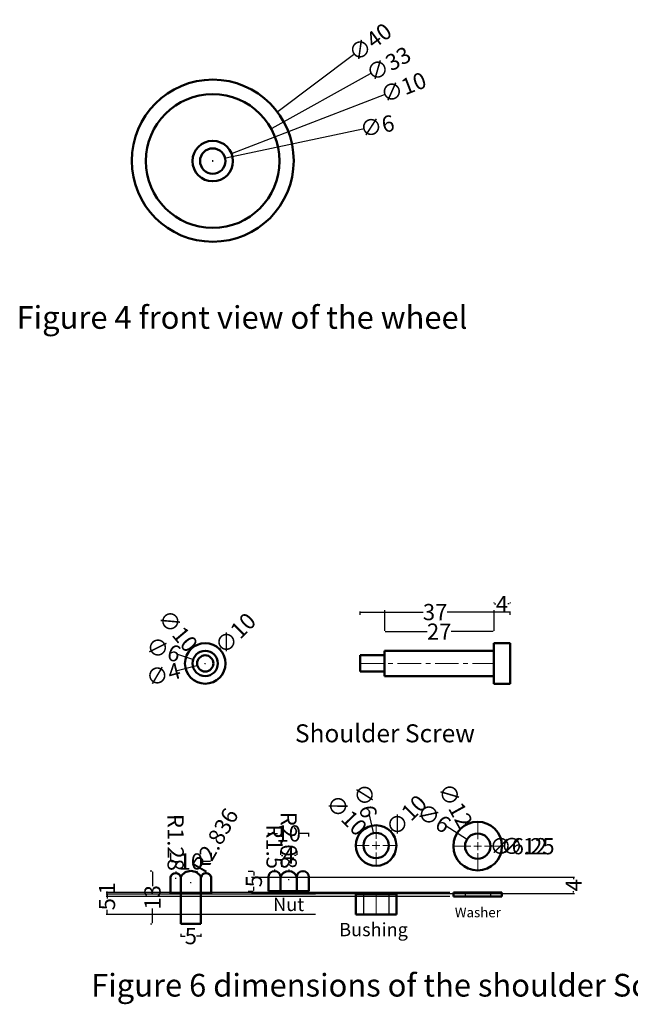
# Model space of a CAD drawing. Units: millimetres. Extents: x 1183 to 1513, y 471 to 941.
# Tile 1 of 3: x 1210 to 1360, y 471 to 714. Entities that reach past the tile are written whole.
import ezdxf

# ---------------------------------------------------------------- set-up
doc = ezdxf.new("R2010")
doc.units = ezdxf.units.MM
doc.header["$LTSCALE"] = 1.4
doc.header["$MEASUREMENT"] = 0
doc.linetypes.add('CENTER', pattern=[50.8, 31.75, -6.35, 6.35, -6.35])
doc.linetypes.add('HIDDEN', pattern=[9.525, 6.35, -3.175])
for name, color, linetype, lineweight in [('M-CNTR', 1, 'CENTER', 18), ('M-DIMS', 2, 'Continuous', 25), ('M-HIDN', 4, 'HIDDEN', 25), ('M-OUTL', 7, 'Continuous', 50), ('M-TEXT', 3, 'Continuous', 25)]:
    doc.layers.add(name, color=color, linetype=linetype, lineweight=lineweight)
doc.styles.get("Standard").update_dxf_attribs({"font": 'arial.ttf'})
doc.dimstyles.get("Standard").update_dxf_attribs({"dimtxt": 4, "dimasz": 0.18, "dimexe": 0.18, "dimexo": 10, "dimgap": 0.09, "dimtad": 0, "dimdec": 0, "dimzin": 0, "dimdsep": 46, "dimtxsty": 'Standard', "dimcen": 0.09, "dimadec": 0, "dimazin": 0, "dimtfac": 1, "dimtdec": 0, "dimtofl": 0, "dimtmove": 0, "dimatfit": 3, "dimfxl": 1, "dimtolj": 1, "dimtzin": 0, "dimarcsym": 0})

# ---------------------------------------------------------------- blocks, each defined once
blk = doc.blocks.new('*D22')
at = {"layer": 'Defpoints', "color": 0, "lineweight": 140, "ltscale": 0.13, "transparency": 16777216}
for p in [(1254.21, 678.48), (1260.33, 679.78)]:
    blk.add_point(p, dxfattribs=at)
at = {"layer": 'M-DIMS', "color": 0, "lineweight": -2, "ltscale": 0.13, "transparency": 16777216}
for p, q in [((1294.37, 687.04), (1260.5, 679.82)), ((1257.18, 679.13), (1257.36, 679.13)), ((1257.27, 679.04), (1257.27, 679.22))]:
    blk.add_line(p, q, dxfattribs=at)
at = {"layer": 'M-DIMS', "color": 0, "lineweight": 140, "ltscale": 0.13, "transparency": 16777216}
blk.add_solid([(1260.5, 679.85), (1260.51, 679.79), (1260.33, 679.78)], dxfattribs=at)
at = {"layer": 'M-DIMS', "color": 0, "ltscale": 0.13, "transparency": 16777216, "insert": (1297.87, 687.78), "char_height": 4, "attachment_point": 5, "rotation": 12.0342}
blk.add_mtext('\\A1;∅6', dxfattribs=at)
blk = doc.blocks.new('*D23')
at = {"layer": 'Defpoints', "color": 0, "lineweight": 140, "ltscale": 0.13, "transparency": 16777216}
for p in [(1261.94, 680.93), (1252.61, 677.33)]:
    blk.add_point(p, dxfattribs=at)
at = {"layer": 'M-DIMS', "color": 0, "lineweight": -2, "ltscale": 0.13, "transparency": 16777216}
for p, q in [((1299.56, 695.46), (1262.1, 680.99)), ((1257.18, 679.13), (1257.36, 679.13)), ((1257.27, 679.04), (1257.27, 679.22))]:
    blk.add_line(p, q, dxfattribs=at)
at = {"layer": 'M-DIMS', "color": 0, "lineweight": 140, "ltscale": 0.13, "transparency": 16777216}
blk.add_solid([(1262.09, 681.02), (1262.11, 680.97), (1261.94, 680.93)], dxfattribs=at)
at = {"layer": 'M-DIMS', "color": 0, "ltscale": 0.13, "transparency": 16777216, "insert": (1304.34, 697.31), "char_height": 4, "attachment_point": 5, "rotation": 21.1163}
blk.add_mtext('\\A1;∅10', dxfattribs=at)
blk = doc.blocks.new('*D24')
at = {"layer": 'Defpoints', "color": 0, "lineweight": 140, "ltscale": 0.13, "transparency": 16777216}
for p in [(1271.71, 687.11), (1242.83, 671.15)]:
    blk.add_point(p, dxfattribs=at)
at = {"layer": 'M-DIMS', "color": 0, "lineweight": -2, "ltscale": 0.13, "transparency": 16777216}
for p, q in [((1296.18, 700.62), (1271.87, 687.19)), ((1257.18, 679.13), (1257.36, 679.13)), ((1257.27, 679.04), (1257.27, 679.22))]:
    blk.add_line(p, q, dxfattribs=at)
at = {"layer": 'M-DIMS', "color": 0, "lineweight": 140, "ltscale": 0.13, "transparency": 16777216}
blk.add_solid([(1271.86, 687.22), (1271.89, 687.17), (1271.71, 687.11)], dxfattribs=at)
at = {"layer": 'M-DIMS', "color": 0, "ltscale": 0.13, "transparency": 16777216, "insert": (1300.67, 703.1), "char_height": 4, "attachment_point": 5, "rotation": 28.9156}
blk.add_mtext('\\A1;∅33', dxfattribs=at)
blk = doc.blocks.new('*D25')
at = {"layer": 'Defpoints', "color": 0, "lineweight": 140, "ltscale": 0.13, "transparency": 16777216}
for p in [(1273.25, 691.25), (1241.29, 667.19)]:
    blk.add_point(p, dxfattribs=at)
at = {"layer": 'M-DIMS', "color": 0, "lineweight": -2, "ltscale": 0.13, "transparency": 16777216}
for p, q in [((1292.01, 705.37), (1273.39, 691.36)), ((1257.18, 679.22), (1257.36, 679.22)), ((1257.27, 679.13), (1257.27, 679.31))]:
    blk.add_line(p, q, dxfattribs=at)
at = {"layer": 'M-DIMS', "color": 0, "lineweight": 140, "ltscale": 0.13, "transparency": 16777216}
blk.add_solid([(1273.37, 691.38), (1273.41, 691.33), (1273.25, 691.25)], dxfattribs=at)
at = {"layer": 'M-DIMS', "color": 0, "ltscale": 0.13, "transparency": 16777216, "insert": (1296.11, 708.45), "char_height": 4, "attachment_point": 5, "rotation": 36.9731}
blk.add_mtext('\\A1;∅40', dxfattribs=at)
blk = doc.blocks.new('*D30')
at = {"layer": 'Defpoints', "color": 0, "lineweight": 140, "ltscale": 0.13, "transparency": 16777216}
for p in [(1252.21, 559), (1258.63, 551.33)]:
    blk.add_point(p, dxfattribs=at)
at = {"layer": 'M-DIMS', "color": 0, "lineweight": -2, "ltscale": 0.13, "transparency": 16777216}
for p, q in [((1251.98, 559.27), (1252.1, 559.13)), ((1255.33, 555.16), (1255.51, 555.16)), ((1255.42, 555.07), (1255.42, 555.25))]:
    blk.add_line(p, q, dxfattribs=at)
at = {"layer": 'M-DIMS', "color": 0, "lineweight": 140, "ltscale": 0.13, "transparency": 16777216}
blk.add_solid([(1252.12, 559.15), (1252.07, 559.11), (1252.21, 559)], dxfattribs=at)
at = {"layer": 'M-DIMS', "color": 0, "ltscale": 0.13, "transparency": 16777216, "insert": (1248.69, 563.2), "char_height": 4, "attachment_point": 5, "rotation": 309.9179}
blk.add_mtext('\\A1;∅10', dxfattribs=at)
blk = doc.blocks.new('*D31')
at = {"layer": 'Defpoints', "color": 0, "lineweight": 140, "ltscale": 0.13, "transparency": 16777216}
for p in [(1252.45, 556.14), (1258.39, 554.19)]:
    blk.add_point(p, dxfattribs=at)
at = {"layer": 'M-DIMS', "color": 0, "lineweight": -2, "ltscale": 0.13, "transparency": 16777216}
for p, q in [((1248.54, 557.42), (1252.28, 556.19)), ((1255.33, 555.16), (1255.51, 555.16)), ((1255.42, 555.07), (1255.42, 555.25))]:
    blk.add_line(p, q, dxfattribs=at)
at = {"layer": 'M-DIMS', "color": 0, "lineweight": 140, "ltscale": 0.13, "transparency": 16777216}
blk.add_solid([(1252.29, 556.22), (1252.27, 556.16), (1252.45, 556.14)], dxfattribs=at)
at = {"layer": 'M-DIMS', "color": 0, "ltscale": 0.13, "transparency": 16777216, "insert": (1245.15, 558.54), "char_height": 4, "attachment_point": 5, "rotation": 341.803}
blk.add_mtext('\\A1;∅6', dxfattribs=at)
blk = doc.blocks.new('*D32')
at = {"layer": 'Defpoints', "color": 0, "lineweight": 140, "ltscale": 0.13, "transparency": 16777216}
for p in [(1253.48, 554.67), (1257.36, 555.66)]:
    blk.add_point(p, dxfattribs=at)
at = {"layer": 'M-DIMS', "color": 0, "lineweight": -2, "ltscale": 0.13, "transparency": 16777216}
for p, q in [((1248.52, 553.4), (1253.31, 554.62)), ((1255.33, 555.16), (1255.51, 555.16)), ((1255.42, 555.07), (1255.42, 555.25))]:
    blk.add_line(p, q, dxfattribs=at)
at = {"layer": 'M-DIMS', "color": 0, "lineweight": 140, "ltscale": 0.13, "transparency": 16777216}
blk.add_solid([(1253.3, 554.65), (1253.32, 554.59), (1253.48, 554.67)], dxfattribs=at)
at = {"layer": 'M-DIMS', "color": 0, "ltscale": 0.13, "transparency": 16777216, "insert": (1245.07, 552.51), "char_height": 4, "attachment_point": 5, "rotation": 14.3659}
blk.add_mtext('\\A1;∅4', dxfattribs=at)
blk = doc.blocks.new('*D33')
at = {"layer": 'Defpoints', "color": 0, "lineweight": 140, "ltscale": 0.13, "transparency": 16777216}
for p in [(1330.68, 569.83), (1326.68, 560.16), (1330.68, 560.16)]:
    blk.add_point(p, dxfattribs=at)
at = {"layer": 'M-DIMS', "color": 0, "lineweight": -2, "ltscale": 0.13, "transparency": 16777216}
for p, q in [((1326.68, 570.16), (1326.68, 570.01)), ((1326.86, 569.83), (1327.21, 569.83)), ((1330.5, 569.83), (1330.16, 569.83)), ((1330.68, 570.16), (1330.68, 570.01))]:
    blk.add_line(p, q, dxfattribs=at)
at = {"layer": 'M-DIMS', "color": 0, "lineweight": 140, "ltscale": 0.13, "transparency": 16777216}
for points in [[(1326.86, 569.86), (1326.86, 569.8), (1326.68, 569.83)], [(1330.5, 569.86), (1330.5, 569.8), (1330.68, 569.83)]]:
    blk.add_solid(points, dxfattribs=at)
at = {"layer": 'M-DIMS', "color": 0, "ltscale": 0.13, "transparency": 16777216, "insert": (1328.68, 569.83), "char_height": 4, "attachment_point": 5}
blk.add_mtext('\\A1;4', dxfattribs=at)
blk = doc.blocks.new('*D34')
at = {"layer": 'Defpoints', "color": 0, "lineweight": 140, "ltscale": 0.13, "transparency": 16777216}
for p in [(1330.68, 567.83), (1293.68, 557.16), (1330.68, 557.16)]:
    blk.add_point(p, dxfattribs=at)
at = {"layer": 'M-DIMS', "color": 0, "lineweight": -2, "ltscale": 0.13, "transparency": 16777216}
for p, q in [((1293.68, 567.16), (1293.68, 568.01)), ((1293.86, 567.83), (1309.23, 567.83)), ((1330.5, 567.83), (1315.14, 567.83)), ((1330.68, 567.16), (1330.68, 568.01))]:
    blk.add_line(p, q, dxfattribs=at)
at = {"layer": 'M-DIMS', "color": 0, "lineweight": 140, "ltscale": 0.13, "transparency": 16777216}
for points in [[(1293.86, 567.86), (1293.86, 567.8), (1293.68, 567.83)], [(1330.5, 567.86), (1330.5, 567.8), (1330.68, 567.83)]]:
    blk.add_solid(points, dxfattribs=at)
at = {"layer": 'M-DIMS', "color": 0, "ltscale": 0.13, "transparency": 16777216, "insert": (1312.18, 567.83), "char_height": 4, "attachment_point": 5}
blk.add_mtext('\\A1;37', dxfattribs=at)
blk = doc.blocks.new('*D35')
at = {"layer": 'Defpoints', "color": 0, "lineweight": 140, "ltscale": 0.13, "transparency": 16777216}
for p in [(1326.68, 563.01), (1299.68, 558.29), (1326.68, 558.29)]:
    blk.add_point(p, dxfattribs=at)
at = {"layer": 'M-DIMS', "color": 0, "lineweight": -2, "ltscale": 0.13, "transparency": 16777216}
for p, q in [((1299.68, 568.29), (1299.68, 563.19)), ((1326.68, 568.29), (1326.68, 563.19)), ((1299.86, 563.01), (1310.2, 563.01)), ((1326.5, 563.01), (1316.17, 563.01))]:
    blk.add_line(p, q, dxfattribs=at)
at = {"layer": 'M-DIMS', "color": 0, "lineweight": 140, "ltscale": 0.13, "transparency": 16777216}
for points in [[(1299.86, 563.04), (1299.86, 562.98), (1299.68, 563.01)], [(1326.5, 563.04), (1326.5, 562.98), (1326.68, 563.01)]]:
    blk.add_solid(points, dxfattribs=at)
at = {"layer": 'M-DIMS', "color": 0, "ltscale": 0.13, "transparency": 16777216, "insert": (1313.18, 563.01), "char_height": 4, "attachment_point": 5}
blk.add_mtext('\\A1;27', dxfattribs=at)
blk = doc.blocks.new('*D36')
at = {"layer": 'Defpoints', "color": 0, "lineweight": 140, "ltscale": 0.13, "transparency": 16777216}
for p in [(1256.87, 506.3), (1246.87, 498.43), (1256.87, 498.43)]:
    blk.add_point(p, dxfattribs=at)
at = {"layer": 'M-DIMS', "color": 0, "lineweight": -2, "ltscale": 0.13, "transparency": 16777216}
for p, q in [((1246.87, 508.43), (1246.87, 506.48)), ((1256.87, 508.43), (1256.87, 506.48)), ((1247.05, 506.3), (1249.11, 506.3)), ((1256.69, 506.3), (1254.63, 506.3))]:
    blk.add_line(p, q, dxfattribs=at)
at = {"layer": 'M-DIMS', "color": 0, "lineweight": 140, "ltscale": 0.13, "transparency": 16777216}
for points in [[(1247.05, 506.33), (1247.05, 506.27), (1246.87, 506.3)], [(1256.69, 506.33), (1256.69, 506.27), (1256.87, 506.3)]]:
    blk.add_solid(points, dxfattribs=at)
at = {"layer": 'M-DIMS', "color": 0, "ltscale": 0.13, "transparency": 16777216, "insert": (1251.87, 506.3), "char_height": 4, "attachment_point": 5}
blk.add_mtext('\\A1;10', dxfattribs=at)
blk = doc.blocks.new('*D37')
at = {"layer": 'Defpoints', "color": 0, "lineweight": 140, "ltscale": 0.13, "transparency": 16777216}
for p in [(1249.37, 498.43), (1254.37, 498.43), (1254.37, 487.87)]:
    blk.add_point(p, dxfattribs=at)
at = {"layer": 'M-DIMS', "color": 0, "lineweight": -2, "ltscale": 0.13, "transparency": 16777216}
for p, q in [((1249.37, 488.43), (1249.37, 487.69)), ((1254.37, 488.43), (1254.37, 487.69)), ((1249.55, 487.87), (1250.46, 487.87)), ((1254.19, 487.87), (1253.29, 487.87))]:
    blk.add_line(p, q, dxfattribs=at)
at = {"layer": 'M-DIMS', "color": 0, "lineweight": 140, "ltscale": 0.13, "transparency": 16777216}
for points in [[(1249.55, 487.9), (1249.55, 487.84), (1249.37, 487.87)], [(1254.19, 487.9), (1254.19, 487.84), (1254.37, 487.87)]]:
    blk.add_solid(points, dxfattribs=at)
at = {"layer": 'M-DIMS', "color": 0, "ltscale": 0.13, "transparency": 16777216, "insert": (1251.87, 487.87), "char_height": 4, "attachment_point": 5}
blk.add_mtext('\\A1;5', dxfattribs=at)
blk = doc.blocks.new('*D38')
at = {"layer": 'Defpoints', "color": 0, "lineweight": 140, "ltscale": 0.13, "transparency": 16777216}
for p in [(1278.03, 507.78), (1274.03, 498.93), (1278.03, 498.93)]:
    blk.add_point(p, dxfattribs=at)
at = {"layer": 'M-DIMS', "color": 0, "lineweight": -2, "ltscale": 0.13, "transparency": 16777216}
for p, q in [((1274.03, 508.93), (1274.03, 507.96)), ((1278.03, 508.93), (1278.03, 507.96)), ((1274.21, 507.78), (1274.56, 507.78)), ((1277.85, 507.78), (1277.5, 507.78))]:
    blk.add_line(p, q, dxfattribs=at)
at = {"layer": 'M-DIMS', "color": 0, "lineweight": 140, "ltscale": 0.13, "transparency": 16777216}
for points in [[(1274.21, 507.81), (1274.21, 507.75), (1274.03, 507.78)], [(1277.85, 507.81), (1277.85, 507.75), (1278.03, 507.78)]]:
    blk.add_solid(points, dxfattribs=at)
at = {"layer": 'M-DIMS', "color": 0, "ltscale": 0.13, "transparency": 16777216, "insert": (1276.03, 507.78), "char_height": 4, "attachment_point": 5}
blk.add_mtext('\\A1;4', dxfattribs=at)
blk = doc.blocks.new('*D39')
at = {"layer": 'Defpoints', "color": 0, "lineweight": 140, "ltscale": 0.13, "transparency": 16777216}
for p in [(1294.12, 513.81), (1301.09, 506.64)]:
    blk.add_point(p, dxfattribs=at)
at = {"layer": 'M-DIMS', "color": 0, "lineweight": -2, "ltscale": 0.13, "transparency": 16777216}
for p, q in [((1293.87, 514.07), (1293.99, 513.94)), ((1297.61, 510.13), (1297.61, 510.31)), ((1297.52, 510.22), (1297.7, 510.22))]:
    blk.add_line(p, q, dxfattribs=at)
at = {"layer": 'M-DIMS', "color": 0, "lineweight": 140, "ltscale": 0.13, "transparency": 16777216}
blk.add_solid([(1294.01, 513.96), (1293.97, 513.92), (1294.12, 513.81)], dxfattribs=at)
at = {"layer": 'M-DIMS', "color": 0, "ltscale": 0.13, "transparency": 16777216, "insert": (1290.29, 517.74), "char_height": 4, "attachment_point": 5, "rotation": 314.2278}
blk.add_mtext('\\A1;∅10', dxfattribs=at)
blk = doc.blocks.new('*D40')
at = {"layer": 'Defpoints', "color": 0, "lineweight": 140, "ltscale": 0.13, "transparency": 16777216}
for p in [(1296.9, 513.27), (1298.31, 507.18)]:
    blk.add_point(p, dxfattribs=at)
at = {"layer": 'M-DIMS', "color": 0, "lineweight": -2, "ltscale": 0.13, "transparency": 16777216}
for p, q in [((1295.86, 517.78), (1296.86, 513.44)), ((1297.61, 510.13), (1297.61, 510.31)), ((1297.52, 510.22), (1297.7, 510.22))]:
    blk.add_line(p, q, dxfattribs=at)
at = {"layer": 'M-DIMS', "color": 0, "lineweight": 140, "ltscale": 0.13, "transparency": 16777216}
blk.add_solid([(1296.89, 513.45), (1296.83, 513.44), (1296.9, 513.27)], dxfattribs=at)
at = {"layer": 'M-DIMS', "color": 0, "ltscale": 0.13, "transparency": 16777216, "insert": (1295.05, 521.26), "char_height": 4, "attachment_point": 5, "rotation": 283.0221}
blk.add_mtext('\\A1;∅6', dxfattribs=at)
blk = doc.blocks.new('*D41')
at = {"layer": 'Defpoints', "color": 0, "lineweight": 140, "ltscale": 0.13, "transparency": 16777216}
for p in [(1319.81, 515.34), (1325.57, 504.81)]:
    blk.add_point(p, dxfattribs=at)
at = {"layer": 'M-DIMS', "color": 0, "lineweight": -2, "ltscale": 0.13, "transparency": 16777216}
for p, q in [((1319.64, 515.65), (1319.72, 515.49)), ((1322.6, 510.07), (1322.78, 510.07)), ((1322.69, 509.98), (1322.69, 510.16))]:
    blk.add_line(p, q, dxfattribs=at)
at = {"layer": 'M-DIMS', "color": 0, "lineweight": 140, "ltscale": 0.13, "transparency": 16777216}
blk.add_solid([(1319.75, 515.51), (1319.7, 515.48), (1319.81, 515.34)], dxfattribs=at)
at = {"layer": 'M-DIMS', "color": 0, "ltscale": 0.13, "transparency": 16777216, "insert": (1317.18, 520.13), "char_height": 4, "attachment_point": 5, "rotation": 298.7027}
blk.add_mtext('\\A1;∅12', dxfattribs=at)
blk = doc.blocks.new('*D42')
at = {"layer": 'Defpoints', "color": 0, "lineweight": 140, "ltscale": 0.13, "transparency": 16777216}
for p in [(1320.06, 511.76), (1325.32, 508.38)]:
    blk.add_point(p, dxfattribs=at)
at = {"layer": 'M-DIMS', "color": 0, "lineweight": -2, "ltscale": 0.13, "transparency": 16777216}
for p, q in [((1314.88, 515.09), (1319.91, 511.86)), ((1322.6, 510.07), (1322.78, 510.07)), ((1322.69, 509.98), (1322.69, 510.16))]:
    blk.add_line(p, q, dxfattribs=at)
at = {"layer": 'M-DIMS', "color": 0, "lineweight": 140, "ltscale": 0.13, "transparency": 16777216}
blk.add_solid([(1319.93, 511.88), (1319.89, 511.83), (1320.06, 511.76)], dxfattribs=at)
at = {"layer": 'M-DIMS', "color": 0, "ltscale": 0.13, "transparency": 16777216, "insert": (1311.87, 517.02), "char_height": 4, "attachment_point": 5, "rotation": 327.2927}
blk.add_mtext('\\A1;∅6', dxfattribs=at)
blk = doc.blocks.new('*D43')
at = {"layer": 'Defpoints', "color": 0, "lineweight": 140, "ltscale": 0.13, "transparency": 16777216}
for p in [(1281.03, 513.21), (1271.03, 502.43), (1281.03, 502.43)]:
    blk.add_point(p, dxfattribs=at)
at = {"layer": 'M-DIMS', "color": 0, "lineweight": -2, "ltscale": 0.13, "transparency": 16777216}
for p, q in [((1271.03, 512.43), (1271.03, 513.39)), ((1271.21, 513.21), (1273.27, 513.21)), ((1280.85, 513.21), (1278.79, 513.21)), ((1281.03, 512.43), (1281.03, 513.39))]:
    blk.add_line(p, q, dxfattribs=at)
at = {"layer": 'M-DIMS', "color": 0, "lineweight": 140, "ltscale": 0.13, "transparency": 16777216}
for points in [[(1271.21, 513.24), (1271.21, 513.18), (1271.03, 513.21)], [(1280.85, 513.24), (1280.85, 513.18), (1281.03, 513.21)]]:
    blk.add_solid(points, dxfattribs=at)
at = {"layer": 'M-DIMS', "color": 0, "ltscale": 0.13, "transparency": 16777216, "insert": (1276.03, 513.21), "char_height": 4, "attachment_point": 5}
blk.add_mtext('\\A1;10', dxfattribs=at)
blk = doc.blocks.new('*D44')
at = {"layer": 'Defpoints', "color": 0, "lineweight": 140, "ltscale": 1.4, "transparency": 16777216}
for p in [(1267.43, 503.93), (1276.03, 503.93), (1276.03, 498.93)]:
    blk.add_point(p, dxfattribs=at)
at = {"layer": 'M-DIMS', "color": 0, "lineweight": -2, "ltscale": 1.4, "transparency": 16777216}
for p, q in [((1266.03, 503.93), (1267.25, 503.93)), ((1267.43, 503.75), (1267.43, 502.85)), ((1266.03, 498.93), (1267.25, 498.93)), ((1267.43, 499.11), (1267.43, 500.02))]:
    blk.add_line(p, q, dxfattribs=at)
at = {"layer": 'M-DIMS', "color": 0, "lineweight": 140, "ltscale": 1.4, "transparency": 16777216}
for points in [[(1267.4, 503.75), (1267.46, 503.75), (1267.43, 503.93)], [(1267.4, 499.11), (1267.46, 499.11), (1267.43, 498.93)]]:
    blk.add_solid(points, dxfattribs=at)
at = {"layer": 'M-DIMS', "color": 0, "ltscale": 1.4, "transparency": 16777216, "insert": (1267.43, 501.43), "char_height": 4, "attachment_point": 5, "rotation": 90}
blk.add_mtext('\\A1;5', dxfattribs=at)
blk = doc.blocks.new('*D45')
at = {"layer": 'Defpoints', "color": 0, "lineweight": 140, "ltscale": 1.4, "transparency": 16777216}
for p in [(1251.86, 503.95), (1242.4, 490.93), (1251.87, 490.93)]:
    blk.add_point(p, dxfattribs=at)
at = {"layer": 'M-DIMS', "color": 0, "lineweight": -2, "ltscale": 1.4, "transparency": 16777216}
for p, q in [((1241.86, 503.95), (1242.22, 503.95)), ((1242.4, 503.77), (1242.4, 500.21)), ((1242.4, 491.11), (1242.4, 494.68)), ((1241.87, 490.93), (1242.22, 490.93))]:
    blk.add_line(p, q, dxfattribs=at)
at = {"layer": 'M-DIMS', "color": 0, "lineweight": 140, "ltscale": 1.4, "transparency": 16777216}
for points in [[(1242.37, 503.77), (1242.43, 503.77), (1242.4, 503.95)], [(1242.37, 491.11), (1242.43, 491.11), (1242.4, 490.93)]]:
    blk.add_solid(points, dxfattribs=at)
at = {"layer": 'M-DIMS', "color": 0, "ltscale": 1.4, "transparency": 16777216, "insert": (1242.4, 497.44), "char_height": 4, "attachment_point": 5, "rotation": 90}
blk.add_mtext('\\A1;13', dxfattribs=at)
blk = doc.blocks.new('*D52')
at = {"layer": 'Defpoints', "color": 0, "lineweight": 140, "ltscale": 1.4, "transparency": 16777216}
for p in [(1256.87, 502.43), (1346.38, 502.43), (1256.87, 498.43)]:
    blk.add_point(p, dxfattribs=at)
at = {"layer": 'M-DIMS', "color": 0, "lineweight": -2, "ltscale": 1.4, "transparency": 16777216}
for p, q in [((1266.87, 502.43), (1346.56, 502.43)), ((1346.38, 502.25), (1346.38, 501.91)), ((1266.87, 498.43), (1346.56, 498.43)), ((1346.38, 498.61), (1346.38, 498.96))]:
    blk.add_line(p, q, dxfattribs=at)
at = {"layer": 'M-DIMS', "color": 0, "lineweight": 140, "ltscale": 1.4, "transparency": 16777216}
for points in [[(1346.35, 502.25), (1346.41, 502.25), (1346.38, 502.43)], [(1346.35, 498.61), (1346.41, 498.61), (1346.38, 498.43)]]:
    blk.add_solid(points, dxfattribs=at)
at = {"layer": 'M-DIMS', "color": 0, "ltscale": 1.4, "transparency": 16777216, "insert": (1346.38, 500.43), "char_height": 4, "attachment_point": 5, "rotation": 90}
blk.add_mtext('\\A1;4', dxfattribs=at)
blk = doc.blocks.new('*D53')
at = {"layer": 'Defpoints', "color": 0, "lineweight": 140, "ltscale": 1.4, "transparency": 16777216}
for p in [(1231.17, 498.24), (1292.61, 498.24), (1292.61, 493.24)]:
    blk.add_point(p, dxfattribs=at)
at = {"layer": 'M-DIMS', "color": 0, "lineweight": -2, "ltscale": 1.4, "transparency": 16777216}
for p, q in [((1282.61, 498.24), (1230.99, 498.24)), ((1231.17, 498.06), (1231.17, 497.16)), ((1282.61, 493.24), (1230.99, 493.24)), ((1231.17, 493.42), (1231.17, 494.32))]:
    blk.add_line(p, q, dxfattribs=at)
at = {"layer": 'M-DIMS', "color": 0, "lineweight": 140, "ltscale": 1.4, "transparency": 16777216}
for points in [[(1231.14, 498.06), (1231.2, 498.06), (1231.17, 498.24)], [(1231.14, 493.42), (1231.2, 493.42), (1231.17, 493.24)]]:
    blk.add_solid(points, dxfattribs=at)
at = {"layer": 'M-DIMS', "color": 0, "ltscale": 1.4, "transparency": 16777216, "insert": (1231.17, 495.74), "char_height": 4, "attachment_point": 5, "rotation": 90}
blk.add_mtext('\\A1;5', dxfattribs=at)
blk = doc.blocks.new('*D54')
at = {"layer": 'Defpoints', "color": 0, "lineweight": 140, "ltscale": 1.4, "transparency": 16777216}
for p in [(1231.17, 498.67), (1325.82, 498.67), (1325.82, 497.67)]:
    blk.add_point(p, dxfattribs=at)
at = {"layer": 'M-DIMS', "color": 0, "lineweight": -2, "ltscale": 1.4, "transparency": 16777216}
for p, q in [((1315.82, 498.67), (1230.99, 498.67)), ((1231.17, 498.67), (1231.17, 498.85)), ((1231.17, 497.85), (1231.17, 498.49)), ((1315.82, 497.67), (1230.99, 497.67))]:
    blk.add_line(p, q, dxfattribs=at)
at = {"layer": 'M-DIMS', "color": 0, "lineweight": 140, "ltscale": 1.4, "transparency": 16777216}
for points in [[(1231.14, 498.49), (1231.2, 498.49), (1231.17, 498.67)], [(1231.14, 497.85), (1231.2, 497.85), (1231.17, 497.67)]]:
    blk.add_solid(points, dxfattribs=at)
at = {"layer": 'M-DIMS', "color": 0, "ltscale": 1.4, "transparency": 16777216, "insert": (1231.17, 499.67), "char_height": 4, "attachment_point": 5, "rotation": 90}
blk.add_mtext('\\A1;1', dxfattribs=at)
blk = doc.blocks.new('*D56')
at = {"layer": 'Defpoints', "color": 0, "lineweight": 140, "ltscale": 1.4, "transparency": 16777216}
for p in [(1258.96, 558.7), (1251.88, 551.63)]:
    blk.add_point(p, dxfattribs=at)
at = {"layer": 'M-DIMS', "color": 0, "lineweight": -2, "ltscale": 1.4, "transparency": 16777216}
for p, q in [((1259.21, 558.95), (1259.08, 558.82)), ((1255.33, 555.16), (1255.51, 555.16)), ((1255.42, 555.07), (1255.42, 555.25))]:
    blk.add_line(p, q, dxfattribs=at)
at = {"layer": 'M-DIMS', "color": 0, "lineweight": 140, "ltscale": 1.4, "transparency": 16777216}
blk.add_solid([(1259.06, 558.84), (1259.1, 558.8), (1258.96, 558.7)], dxfattribs=at)
at = {"layer": 'M-DIMS', "color": 0, "ltscale": 1.4, "transparency": 16777216, "insert": (1262.83, 562.57), "char_height": 4, "attachment_point": 5, "rotation": 44.9928}
blk.add_mtext('\\A1;∅10', dxfattribs=at)
blk = doc.blocks.new('*D57')
at = {"layer": 'Defpoints', "color": 0, "lineweight": 140, "ltscale": 1.4, "transparency": 16777216}
for p in [(1253.3, 503.58), (1251.88, 501.12)]:
    blk.add_point(p, dxfattribs=at)
at = {"layer": 'M-DIMS', "color": 0, "lineweight": -2, "ltscale": 1.4, "transparency": 16777216}
for p, q in [((1253.47, 503.89), (1253.38, 503.73)), ((1251.79, 501.12), (1251.97, 501.12)), ((1251.88, 501.03), (1251.88, 501.21))]:
    blk.add_line(p, q, dxfattribs=at)
at = {"layer": 'M-DIMS', "color": 0, "lineweight": 140, "ltscale": 1.4, "transparency": 16777216}
blk.add_solid([(1253.36, 503.75), (1253.41, 503.72), (1253.3, 503.58)], dxfattribs=at)
at = {"layer": 'M-DIMS', "color": 0, "ltscale": 1.4, "transparency": 16777216, "insert": (1257.83, 511.48), "char_height": 4, "attachment_point": 5, "rotation": 60.1717}
blk.add_mtext('\\A1;R2.836', dxfattribs=at)
blk = doc.blocks.new('*D58')
at = {"layer": 'Defpoints', "color": 0, "lineweight": 140, "ltscale": 1.4, "transparency": 16777216}
for p in [(1248.12, 503.42), (1248.12, 502.14)]:
    blk.add_point(p, dxfattribs=at)
at = {"layer": 'M-DIMS', "color": 0, "lineweight": -2, "ltscale": 1.4, "transparency": 16777216}
for p, q in [((1248.12, 503.78), (1248.12, 503.6)), ((1248.03, 502.14), (1248.21, 502.14)), ((1248.12, 502.05), (1248.12, 502.23))]:
    blk.add_line(p, q, dxfattribs=at)
at = {"layer": 'M-DIMS', "color": 0, "lineweight": 140, "ltscale": 1.4, "transparency": 16777216}
blk.add_solid([(1248.15, 503.6), (1248.09, 503.6), (1248.12, 503.42)], dxfattribs=at)
at = {"layer": 'M-DIMS', "color": 0, "ltscale": 1.4, "transparency": 16777216, "insert": (1248.11, 510.99), "char_height": 4, "attachment_point": 5, "rotation": 270.0706}
blk.add_mtext('\\A1;R1.28', dxfattribs=at)
blk = doc.blocks.new('*D59')
at = {"layer": 'Defpoints', "color": 0, "lineweight": 140, "ltscale": 1.4, "transparency": 16777216}
for p in [(1272.53, 503.93), (1272.53, 502.43)]:
    blk.add_point(p, dxfattribs=at)
at = {"layer": 'M-DIMS', "color": 0, "lineweight": -2, "ltscale": 1.4, "transparency": 16777216}
for p, q in [((1272.53, 504.29), (1272.53, 504.11)), ((1272.44, 502.43), (1272.62, 502.43)), ((1272.53, 502.34), (1272.53, 502.52))]:
    blk.add_line(p, q, dxfattribs=at)
at = {"layer": 'M-DIMS', "color": 0, "lineweight": 140, "ltscale": 1.4, "transparency": 16777216}
blk.add_solid([(1272.56, 504.11), (1272.5, 504.11), (1272.53, 503.93)], dxfattribs=at)
at = {"layer": 'M-DIMS', "color": 0, "ltscale": 1.4, "transparency": 16777216, "insert": (1272.53, 509.95), "char_height": 4, "attachment_point": 5, "rotation": 270.0249}
blk.add_mtext('\\A1;R1.5', dxfattribs=at)
blk = doc.blocks.new('*D60')
at = {"layer": 'Defpoints', "color": 0, "lineweight": 140, "ltscale": 1.4, "transparency": 16777216}
for p in [(1276.03, 503.93), (1276.03, 501.85)]:
    blk.add_point(p, dxfattribs=at)
at = {"layer": 'M-DIMS', "color": 0, "lineweight": -2, "ltscale": 1.4, "transparency": 16777216}
for p, q in [((1276.03, 504.29), (1276.03, 504.11)), ((1275.94, 501.85), (1276.12, 501.85)), ((1276.03, 501.76), (1276.03, 501.94))]:
    blk.add_line(p, q, dxfattribs=at)
at = {"layer": 'M-DIMS', "color": 0, "lineweight": 140, "ltscale": 1.4, "transparency": 16777216}
blk.add_solid([(1276.06, 504.11), (1276, 504.11), (1276.03, 503.93)], dxfattribs=at)
at = {"layer": 'M-DIMS', "color": 0, "ltscale": 1.4, "transparency": 16777216, "insert": (1276.03, 511.5), "char_height": 4, "attachment_point": 5, "rotation": 270.0182}
blk.add_mtext('\\A1;R2.08', dxfattribs=at)
blk = doc.blocks.new('*D61')
at = {"layer": 'Defpoints', "color": 0, "lineweight": 140, "ltscale": 1.4, "transparency": 16777216}
for p in [(1301.15, 513.75), (1294.06, 506.7)]:
    blk.add_point(p, dxfattribs=at)
at = {"layer": 'M-DIMS', "color": 0, "lineweight": -2, "ltscale": 1.4, "transparency": 16777216}
for p, q in [((1301.41, 514), (1301.28, 513.88)), ((1297.61, 510.13), (1297.61, 510.31)), ((1297.52, 510.22), (1297.7, 510.22))]:
    blk.add_line(p, q, dxfattribs=at)
at = {"layer": 'M-DIMS', "color": 0, "lineweight": 140, "ltscale": 1.4, "transparency": 16777216}
blk.add_solid([(1301.26, 513.9), (1301.3, 513.86), (1301.15, 513.75)], dxfattribs=at)
at = {"layer": 'M-DIMS', "color": 0, "ltscale": 1.4, "transparency": 16777216, "insert": (1305.04, 517.62), "char_height": 4, "attachment_point": 5, "rotation": 44.8507}
blk.add_mtext('\\A1;∅10', dxfattribs=at)
blk = doc.blocks.new('*D62')
at = {"layer": 'Defpoints', "color": 0, "lineweight": 140, "ltscale": 1.4, "transparency": 16777216}
for p in [(1316.69, 510.08), (1328.69, 510.07)]:
    blk.add_point(p, dxfattribs=at)
at = {"layer": 'M-DIMS', "color": 0, "lineweight": -2, "ltscale": 1.4, "transparency": 16777216}
for p, q in [((1322.6, 510.07), (1322.78, 510.07)), ((1322.69, 509.98), (1322.69, 510.16)), ((1329.05, 510.07), (1328.87, 510.07))]:
    blk.add_line(p, q, dxfattribs=at)
at = {"layer": 'M-DIMS', "color": 0, "lineweight": 140, "ltscale": 1.4, "transparency": 16777216}
blk.add_solid([(1328.87, 510.1), (1328.87, 510.04), (1328.69, 510.07)], dxfattribs=at)
at = {"layer": 'M-DIMS', "color": 0, "ltscale": 1.4, "transparency": 16777216, "insert": (1334.16, 510.07), "char_height": 4, "attachment_point": 5, "rotation": 359.9703}
blk.add_mtext('\\A1;∅12', dxfattribs=at)
blk = doc.blocks.new('*D63')
at = {"layer": 'Defpoints', "color": 0, "lineweight": 140, "ltscale": 1.4, "transparency": 16777216}
for p in [(1319.57, 510.08), (1325.82, 510.07)]:
    blk.add_point(p, dxfattribs=at)
at = {"layer": 'M-DIMS', "color": 0, "lineweight": -2, "ltscale": 1.4, "transparency": 16777216}
for p, q in [((1322.6, 510.07), (1322.78, 510.07)), ((1322.69, 509.98), (1322.69, 510.16)), ((1326.18, 510.07), (1326, 510.07))]:
    blk.add_line(p, q, dxfattribs=at)
at = {"layer": 'M-DIMS', "color": 0, "lineweight": 140, "ltscale": 1.4, "transparency": 16777216}
blk.add_solid([(1326, 510.1), (1326, 510.04), (1325.82, 510.07)], dxfattribs=at)
at = {"layer": 'M-DIMS', "color": 0, "ltscale": 1.4, "transparency": 16777216, "insert": (1333.65, 510.06), "char_height": 4, "attachment_point": 5, "rotation": 359.9406}
blk.add_mtext('\\A1;∅6.25', dxfattribs=at)

msp = doc.modelspace()

# ---------------------------------------------------------------- linework, layer by layer
at = {"layer": 'M-CNTR', "ltscale": 0.13}
msp.add_line((1293.6849, 555.1613), (1326.6849, 555.1613), dxfattribs=at)
at = {"layer": 'M-CNTR', "ltscale": 0.35}
for p, q in [((1297.606, 511.9182), (1297.606, 515.2244)), ((1322.6901, 511.7669), (1322.6901, 516.0731)), ((1297.606, 509.2676), (1297.606, 511.1812)), ((1322.6901, 509.1163), (1322.6901, 511.0299)), ((1292.606, 510.2244), (1295.9122, 510.2244)), ((1296.6492, 510.2244), (1298.5628, 510.2244)), ((1297.606, 505.2244), (1297.606, 508.5306)), ((1299.2998, 510.2244), (1302.606, 510.2244)), ((1316.6901, 510.0731), (1320.9963, 510.0731)), ((1321.7333, 510.0731), (1323.6469, 510.0731)), ((1322.6901, 504.0731), (1322.6901, 508.3793)), ((1324.3839, 510.0731), (1328.6901, 510.0731))]:
    msp.add_line(p, q, dxfattribs=at)
at = {"layer": 'M-CNTR', "ltscale": 0.7}
msp.add_line((1297.606, 498.24), (1297.606, 493.24), dxfattribs=at)
at = {"layer": 'M-HIDN', "ltscale": 0.7}
for p, q in [((1294.481, 498.24), (1294.481, 493.24)), ((1300.731, 498.24), (1300.731, 493.24))]:
    msp.add_line(p, q, dxfattribs=at)
at = {"layer": 'M-HIDN', "ltscale": 0.13}
for p, q in [((1319.5651, 498.6654), (1319.5651, 497.6654)), ((1325.8151, 498.6654), (1325.8151, 497.6654))]:
    msp.add_line(p, q, dxfattribs=at)
at = {"layer": 'M-OUTL', "ltscale": 0.13}
for p, q in [((1326.6849, 560.1613), (1330.6849, 560.1613)), ((1326.6849, 560.1613), (1326.6849, 550.1613)), ((1330.6849, 560.1613), (1330.6849, 550.1613)), ((1293.6849, 557.1613), (1293.6849, 553.1613)), ((1293.6849, 557.1613), (1299.6849, 557.1613)), ((1299.6849, 558.2863), (1326.6849, 558.2863)), ((1299.6849, 558.2863), (1299.6849, 552.0363)), ((1293.6849, 553.1613), (1299.6849, 553.1613)), ((1299.6849, 552.0363), (1326.6849, 552.0363)), ((1326.6849, 550.1613), (1330.6849, 550.1613)), ((1246.8714, 498.4334), (1246.8714, 502.4334)), ((1249.3714, 490.9334), (1249.3714, 502.4334)), ((1254.3714, 490.9334), (1254.3714, 502.4816)), ((1256.8714, 502.4334), (1256.8714, 498.4334)), ((1271.0306, 498.9334), (1271.0306, 502.4334)), ((1274.0306, 502.4334), (1274.0306, 498.9334)), ((1278.0306, 502.4334), (1278.0306, 498.9334)), ((1281.0306, 502.4334), (1281.0306, 498.9334)), ((1246.8714, 498.4334), (1256.8714, 498.4334)), ((1271.0306, 498.9334), (1281.0306, 498.9334)), ((1292.606, 498.24), (1292.606, 493.24)), ((1292.606, 498.24), (1302.606, 498.24)), ((1302.606, 498.24), (1302.606, 493.24)), ((1292.606, 493.24), (1302.606, 493.24)), ((1249.3714, 490.9334), (1254.3714, 490.9334))]:
    msp.add_line(p, q, dxfattribs=at)
at = {"layer": 'M-OUTL', "ltscale": 0.35}
for p, q in [((1316.6901, 498.6654), (1316.6901, 497.6654)), ((1316.6901, 498.6654), (1328.6901, 498.6654)), ((1328.6901, 498.6654), (1328.6901, 497.6654)), ((1316.6901, 497.6654), (1328.6901, 497.6654))]:
    msp.add_line(p, q, dxfattribs=at)
at = {"layer": 'M-OUTL', "ltscale": 0.13}
for centre, radius in [((1257.2708, 679.2188), 20), ((1257.2708, 679.1288), 16.5), ((1255.4204, 555.1613), 5), ((1255.4204, 555.1613), 3.125), ((1255.4204, 555.1613), 2), ((1297.606, 510.2244), 5), ((1297.606, 510.2244), 3.125)]:
    msp.add_circle(centre, radius, dxfattribs=at)
at = {"layer": 'M-OUTL', "ltscale": 2}
for radius in [5, 3.125]:
    msp.add_circle((1257.2708, 679.1288), radius, dxfattribs=at)
at = {"layer": 'M-OUTL', "ltscale": 0.35}
for radius in [6, 3.125]:
    msp.add_circle((1322.6901, 510.0731), radius, dxfattribs=at)
at = {"layer": 'M-OUTL', "ltscale": 0.13}
for centre, radius, start, end in [((1248.1214, 502.1411), 1.2837, 13.161532, 166.838468), ((1251.8843, 501.1184), 2.8362, 28.72832, 152.375316), ((1255.6214, 502.1411), 1.2837, 13.161532, 166.838468), ((1272.5306, 502.4334), 1.5, 0, 180), ((1276.0306, 501.8501), 2.0833, 16.260205, 163.739795), ((1279.5306, 502.4334), 1.5, 0, 180)]:
    msp.add_arc(centre, radius, start, end, dxfattribs=at)

# ---------------------------------------------------------------- texts
at = {"layer": 'M-TEXT', "ltscale": 0.13}
for s, height, p in [('Figure 4 front view of the wheel ', 5.601941, (1208.8339, 637.7405)), ('Shoulder Screw ', 4.43907, (1277.5738, 535.6951)), ('Nut ', 3.28228, (1272.1837, 494.0549)), ('Washer', 2.40974, (1317.0467, 492.5228)), ('  Bushing ', 3.28228, (1286.4858, 487.8463)), ('Figure 6 dimensions of the shoulder Screw,Bolt, Nut,Bushing, and Washer ', 5.601941, (1227.2503, 472.9565))]:
    msp.add_text(s, height=height, dxfattribs=at).set_placement(p)

# ---------------------------------------------------------------- dimensions: what is measured, and where the dimension line sits
at = {"layer": 'M-DIMS', "ltscale": 0.13}
for p1, p2, picture, middle in [((1241.2924, 667.19), (1273.2491, 691.2475), '*D25', (1296.1064, 708.4549)), ((1242.8278, 671.1507), (1271.7138, 687.1068), '*D24', (1300.6714, 703.1026)), ((1252.6065, 677.3274), (1261.935, 680.9301), '*D23', (1304.3386, 697.3062)), ((1254.2144, 678.4772), (1260.3271, 679.7803), '*D22', (1297.8683, 687.7834)), ((1258.3891, 554.1854), (1252.4517, 556.1372), '*D31', (1245.147, 558.5384)), ((1257.3579, 555.6575), (1253.4829, 554.6651), '*D32', (1245.0676, 552.5097)), ((1298.3102, 507.1798), (1296.9019, 513.269), '*D40', (1295.0529, 521.264)), ((1325.3196, 508.3845), (1320.0606, 511.7617), '*D42', (1311.8665, 517.0237))]:
    dim = msp.add_diameter_dim_2p(p1=p1, p2=p2, dimstyle='Standard', override={"dimclrd": 0, "dimclre": 0, "dimclrt": 0}, dxfattribs=at)
    dim.commit()
    dim.dimension.update_dxf_attribs({"geometry": picture, "text_midpoint": middle, "dimtype": 163})
for base, p1, p2, picture, middle in [((1330.6849, 569.8347), (1326.6849, 560.1613), (1330.6849, 560.1613), '*D33', (1328.6849, 569.8347)), ((1330.6849, 567.8347), (1293.6849, 557.1613), (1330.6849, 557.1613), '*D34', (1312.1849, 567.8347)), ((1326.6849, 563.0097), (1299.6849, 558.2863), (1326.6849, 558.2863), '*D35', (1313.1849, 563.0097)), ((1281.0306, 513.2088), (1271.0306, 502.4334), (1281.0306, 502.4334), '*D43', (1276.0306, 513.2088)), ((1278.0306, 507.7845), (1274.0306, 498.9334), (1278.0306, 498.9334), '*D38', (1276.0306, 507.7845)), ((1256.8714, 506.2975), (1246.8714, 498.4334), (1256.8714, 498.4334), '*D36', (1251.8714, 506.2975)), ((1254.3714, 487.8723), (1249.3714, 498.4334), (1254.3714, 498.4334), '*D37', (1251.8714, 487.8723))]:
    dim = msp.add_linear_dim(base=base, p1=p1, p2=p2, dimstyle='Standard', override={"dimclrd": 0, "dimclre": 0, "dimclrt": 0}, dxfattribs=at)
    dim.commit()
    dim.dimension.update_dxf_attribs({"geometry": picture, "text_midpoint": middle})
for p1, p2, picture, middle in [((1258.6288, 551.3265), (1252.212, 558.9961), '*D30', (1248.6929, 563.2022)), ((1325.5717, 504.8104), (1319.8085, 515.3359), '*D41', (1317.1812, 520.1341)), ((1301.0936, 506.6415), (1294.1185, 513.8073), '*D39', (1290.2932, 517.737))]:
    dim = msp.add_diameter_dim_2p(p1=p1, p2=p2, dimstyle='Standard', override={"dimclrd": 0, "dimclre": 0, "dimclrt": 0}, dxfattribs=at)
    dim.commit()
    dim.dimension.update_dxf_attribs({"geometry": picture, "text_midpoint": middle})
at = {"layer": 'M-DIMS', "ltscale": 1.4}
for p1, p2, picture, middle in [((1251.8844, 551.6262), (1258.9564, 558.6964), '*D56', (1262.8347, 562.5737)), ((1294.0613, 506.6981), (1301.1508, 513.7507), '*D61', (1305.0387, 517.6184))]:
    dim = msp.add_diameter_dim_2p(p1=p1, p2=p2, dimstyle='Standard', override={"dimdec": 0, "dimlfac": 1, "dimrnd": 0, "dimzin": 0, "dimdsep": 46, "dimlunit": 2}, dxfattribs=at)
    dim.commit()
    dim.dimension.update_dxf_attribs({"geometry": picture, "text_midpoint": middle, "dimtype": 163})
for center, mpoint, override, picture, middle in [((1251.8843, 501.1184), (1253.2951, 503.5788), {"dimdec": 3, "dimlfac": 1, "dimrnd": 0, "dimzin": 0, "dimdsep": 46, "dimlunit": 2}, '*D57', (1257.8272, 511.4834)), ((1248.1214, 502.1411), (1248.1198, 503.4249), {"dimdec": 2, "dimlfac": 1, "dimrnd": 0, "dimzin": 0, "dimdsep": 46, "dimlunit": 2}, '*D58', (1248.1105, 510.9881)), ((1276.0306, 501.8501), (1276.03, 503.9334), {"dimdec": 2, "dimlfac": 1, "dimrnd": 0, "dimzin": 0, "dimdsep": 46, "dimlunit": 2}, '*D60', (1276.0276, 511.4967)), ((1272.5306, 502.4334), (1272.53, 503.9334), {"dimdec": 1, "dimlfac": 1, "dimrnd": 0, "dimzin": 0, "dimdsep": 46, "dimlunit": 2}, '*D59', (1272.5274, 509.9537))]:
    dim = msp.add_radius_dim(center=center, mpoint=mpoint, dimstyle='Standard', override=override, dxfattribs=at)
    dim.commit()
    dim.dimension.update_dxf_attribs({"geometry": picture, "text_midpoint": middle})
for p1, p2, override, picture, middle in [((1316.6901, 510.0762), (1328.6901, 510.07), {"dimdec": 0, "dimlfac": 1, "dimrnd": 0, "dimzin": 0, "dimdsep": 46, "dimlunit": 2}, '*D62', (1334.1606, 510.0672)), ((1319.5651, 510.0763), (1325.8151, 510.0699), {"dimdec": 2, "dimlfac": 1, "dimrnd": 0, "dimzin": 0, "dimdsep": 46, "dimlunit": 2}, '*D63', (1333.6512, 510.0617))]:
    dim = msp.add_diameter_dim_2p(p1=p1, p2=p2, dimstyle='Standard', override=override, dxfattribs=at)
    dim.commit()
    dim.dimension.update_dxf_attribs({"geometry": picture, "text_midpoint": middle})
for base, p1, p2, override, picture, middle in [((1242.4047, 490.9334), (1251.857, 503.9544), (1251.8714, 490.9334), {"dimclrd": 0, "dimclre": 0, "dimclrt": 0}, '*D45', (1242.4047, 497.4439)), ((1267.4274, 503.9334), (1276.0306, 498.9334), (1276.0306, 503.9334), {"dimclrd": 0, "dimclre": 0, "dimclrt": 0}, '*D44', (1267.4274, 501.4334)), ((1231.1714, 498.6654), (1325.8151, 497.6654), (1325.8151, 498.6654), {"dimdec": 0, "dimlfac": 1, "dimrnd": 0, "dimzin": 0, "dimdsep": 46, "dimlunit": 2}, '*D54', (1231.1714, 499.6721)), ((1346.3849, 502.4334), (1256.8714, 498.4334), (1256.8714, 502.4334), {"dimdec": 0, "dimlfac": 1, "dimrnd": 0, "dimzin": 0, "dimdsep": 46, "dimlunit": 2}, '*D52', (1346.3849, 500.4334)), ((1231.1714, 498.24), (1292.606, 493.24), (1292.606, 498.24), {"dimdec": 0, "dimlfac": 1, "dimrnd": 0, "dimzin": 0, "dimdsep": 46, "dimlunit": 2}, '*D53', (1231.1714, 495.74))]:
    dim = msp.add_linear_dim(base=base, p1=p1, p2=p2, angle=90, dimstyle='Standard', override=override, dxfattribs=at)
    dim.commit()
    dim.dimension.update_dxf_attribs({"geometry": picture, "text_midpoint": middle})

doc.saveas('drawing.dxf')
